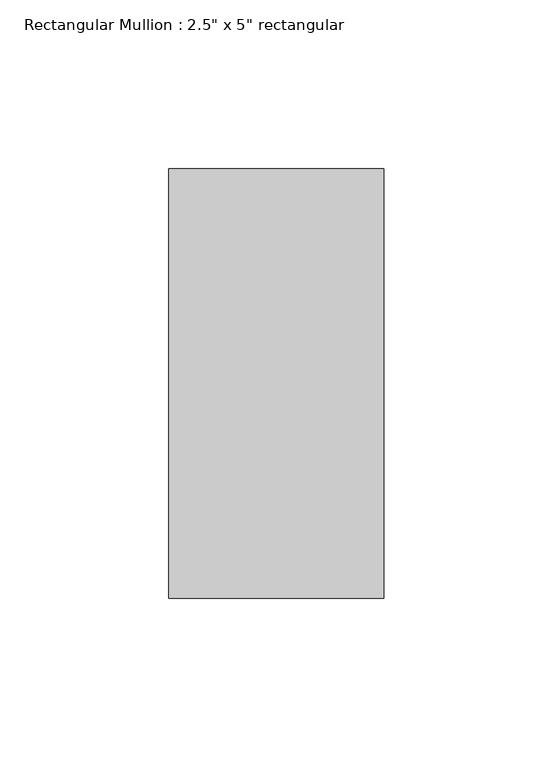
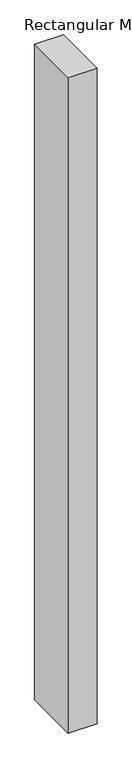
"""IFC4 building model written with IfcOpenShell, lengths in millimetres: member geometry."""

from ifc_helpers import new_model, si_unit, frame, origin, place, context, project, spatial, polyline, outline, extrude, source, transform, mapped, element, save


def member_4491d118(model_context):
    return source(origin(), model_context, "Body", "SweptSolid", [
        extrude(outline(polyline([(0.0, 63.5), (0.0, -63.5), (-63.5, -63.5), (-63.5, 63.5), (0.0, 63.5)])), frame((0.0, 0.0, -1524.0), z_axis=(0.0, 0.0, 1.0), x_axis=(1.0, 0.0, 0.0)), (0.0, 0.0, 1.0), 1524.0),
    ])


if __name__ == "__main__":
    model = new_model("IFC4")
    model_context = context("Model", 3, world=origin())
    ifc_project = project(units=[si_unit("LENGTHUNIT", "METRE", prefix="MILLI")], contexts=[model_context])
    site = spatial("IfcSite", under=ifc_project)
    building = spatial("IfcBuilding", under=site)
    placement = place(None, origin())
    member_shape = member_4491d118(model_context)
    element("IfcMember", 1, ObjectType="Rectangular Mullion : 2.5\" x 5\" rectangular", at=placement, inside=building, context=model_context, shape_type="MappedRepresentation", body=[
        mapped(member_shape, transform((0.0, 0.0, 0.0), x_axis=(1.0, 0.0, 0.0), y_axis=(0.0, 1.0, 0.0), z_axis=(0.0, 0.0, 1.0))),
    ])
    save(model, "model.ifc")

# Revit data of these elements
# Type "Rectangular Mullion : 2.5\" x 5\" rectangular"
#   built-in parameter 1007304 = 0.416667 (stored number, unit not read)
#   built-in parameter 1007301 = 0.104167 (stored number, unit not read)
#   built-in parameter 1007300 = 0.104167 (stored number, unit not read)
# Element 1 (IfcMember, "Rectangular Mullion : 2.5\" x 5\" rectangular")
#   Materials on its faces: "Aluminum"
# Materials
#   "Aluminum": class "Metal", colour RGB 247 247 247, transparency 0, Description = "Aluminum 6061", Cost = 0
